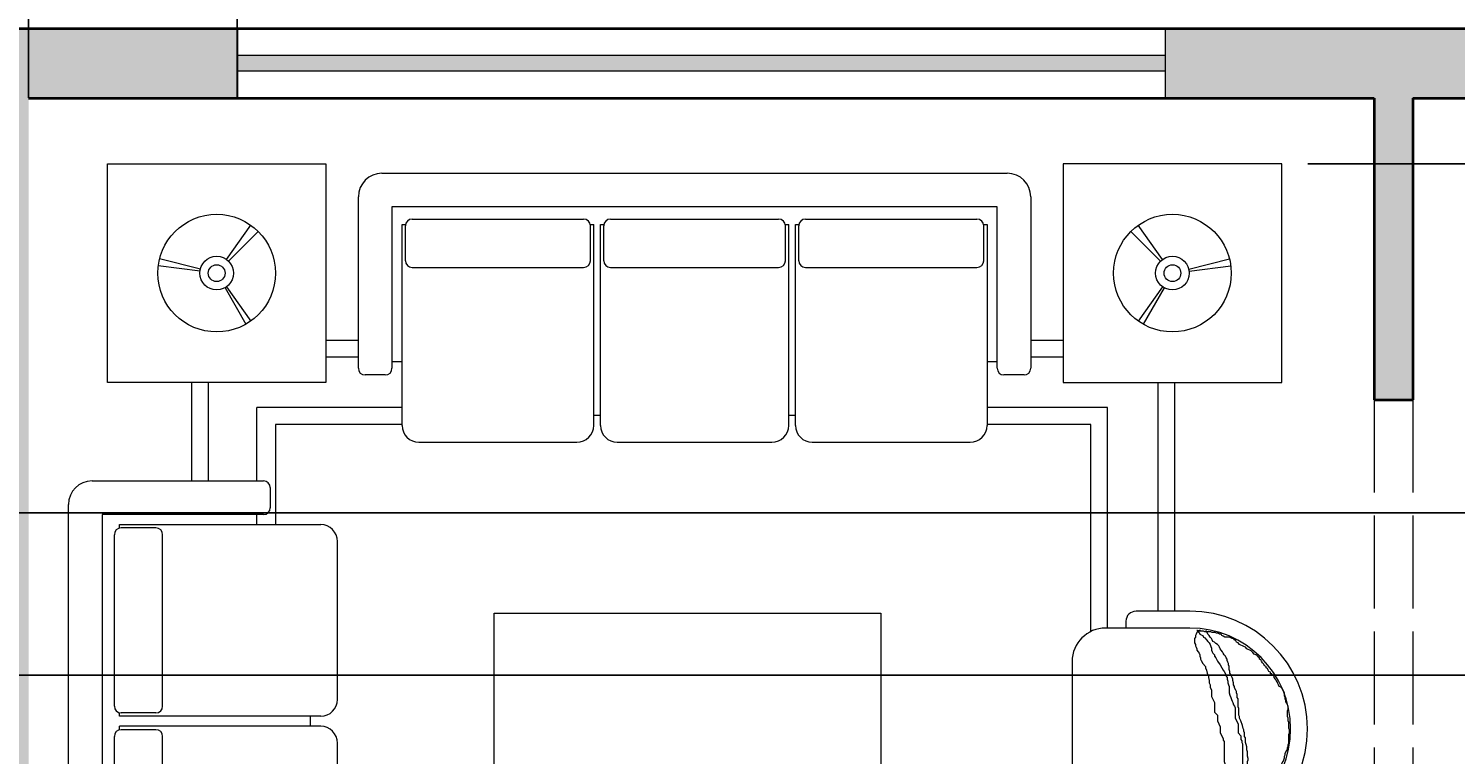
# Model space of a CAD drawing. Units: inches. Extents: x 2330 to 3943, y 1763 to 3461.
# Tile 29 of 40: x 3097 to 3281, y 3069 to 3163. Entities that reach past the tile are written whole.
import ezdxf

# ---------------------------------------------------------------- set-up
doc = ezdxf.new("R2010")
doc.units = ezdxf.units.IN
doc.linetypes.add('ACAD_ISO02W100', pattern=[15, 12, -3])
for name, color, linetype, lineweight in [('A-ANNO-DIMS', 2, 'Continuous', 18), ('A-FURN', 8, 'Continuous', 13), ('A-GLAZ', 4, 'Continuous', 18), ('A-WALL', 7, 'Continuous', 40), ('A-WALL-OVHD', 7, 'ACAD_ISO02W100', 18), ('A-WALL-PATT', 252, 'Continuous', 13)]:
    doc.layers.add(name, color=color, linetype=linetype, lineweight=lineweight)
doc.styles.get("Standard").update_dxf_attribs({"font": 'arial.ttf'})
doc.dimstyles.get("Standard").update_dxf_attribs({"dimtxt": 0.18, "dimasz": 0.18, "dimexe": 0.18, "dimexo": 0.0625, "dimgap": 0.09, "dimtad": 0, "dimtih": 1, "dimtoh": 1, "dimdec": 4, "dimzin": 0, "dimdsep": 46, "dimtxsty": 'Standard', "dimcen": 0.09, "dimadec": 0, "dimazin": 0, "dimtfac": 1, "dimtdec": 4, "dimtofl": 0, "dimtmove": 0, "dimatfit": 3, "dimfxl": 1, "dimtolj": 1, "dimtzin": 0, "dimarcsym": 0})

# ---------------------------------------------------------------- blocks, each defined once
blk = doc.blocks.new('A$C78064EA7')
for p, q in [((932.1, 3320.6), (2792.1, 3320.6)), ((862.1, 2740.6), (862.1, 3250.6)), ((2862.1, 3250.6), (2862.1, 2740.6)), ((962.1, 3220.6), (962.1, 2740.6)), ((2762.1, 3220.6), (962.1, 3220.6)), ((1022.1, 3184.3), (1532.1, 3184.3)), ((1612.1, 3184.3), (2112.1, 3184.3)), ((2192.1, 3184.3), (2702.1, 3184.3)), ((2762.1, 2740.6), (2762.1, 3220.6)), ((469.8, 3064.3), (542.4, 3166)), ((476.1, 3059), (564.4, 3147.3)), ((992.1, 3168.5), (1002.1, 3168.5)), ((992.1, 2570.6), (992.1, 3168.5)), ((1002.1, 3060.6), (1002.1, 3164.3)), ((1551.6, 3168.5), (1562.1, 3168.5)), ((1552.1, 3060.6), (1552.1, 3164.3)), ((1562.1, 2570.6), (1562.1, 3168.5)), ((1582.1, 3168.5), (1592.5, 3168.5)), ((1582.1, 2570.6), (1582.1, 3168.5)), ((1592.1, 3060.6), (1592.1, 3164.3)), ((2131.6, 3168.5), (2142.1, 3168.5)), ((2132.1, 3060.6), (2132.1, 3164.3)), ((2142.1, 2570.6), (2142.1, 3168.5)), ((2162.1, 3168.5), (2172.5, 3168.5)), ((2162.1, 2570.6), (2162.1, 3168.5)), ((2172.1, 3060.6), (2172.1, 3164.3)), ((2721.6, 3168.5), (2732.1, 3168.5)), ((2722.1, 3060.6), (2722.1, 3164.3)), ((2732.1, 3168.5), (2732.1, 2570.6)), ((3248.1, 3059), (3159.7, 3147.3)), ((3254.4, 3064.3), (3181.7, 3166)), ((392.2, 3035.7), (270.9, 3066)), ((3331.9, 3035.7), (3453.2, 3066)), ((391.1, 3029.8), (267.1, 3045.3)), ((1022.1, 3040.6), (1532.1, 3040.6)), ((1612.1, 3040.6), (2112.1, 3040.6)), ((2192.1, 3040.6), (2702.1, 3040.6)), ((3333, 3029.8), (3457.1, 3045.3)), ((465.5, 2980.2), (527.5, 2871.7)), ((469.8, 2982.9), (542.4, 2881.2)), ((3254.4, 2982.9), (3181.7, 2881.2)), ((3258.6, 2980.2), (3196.6, 2871.7)), ((862.1, 2823.6), (765.7, 2823.6)), ((2958.4, 2823.6), (2862.1, 2823.6)), ((862.1, 2773.6), (765.7, 2773.6)), ((962.1, 2760.6), (992.1, 2760.6)), ((2732.1, 2760.6), (2762.1, 2760.6)), ((2958.4, 2773.6), (2862.1, 2773.6)), ((942.1, 2720.6), (882.1, 2720.6)), ((2842.1, 2720.6), (2782.1, 2720.6)), ((365.7, 2698.6), (365.7, 2405.5)), ((415.7, 2698.6), (415.7, 2405.5)), ((3240.7, 2017.9), (3240.7, 2698.6)), ((3290.7, 2017.9), (3290.7, 2698.6)), ((992.1, 2623.6), (560, 2623.6)), ((560, 2405.5), (560, 2623.6)), ((1562.1, 2600.6), (1582.1, 2600.6)), ((2142.1, 2600.6), (2162.1, 2600.6)), ((992.1, 2573.6), (615.7, 2573.6)), ((615.7, 2573.6), (615.7, 2275.5)), ((1042.1, 2520.6), (1512.1, 2520.6)), ((1632.1, 2520.6), (2092.1, 2520.6)), ((2212.1, 2520.6), (2682.1, 2520.6)), ((70, 2405.5), (580, 2405.5)), ((600, 2385.5), (600, 2325.5)), ((0, 1045.5), (0, 2335.5)), ((580, 2305.5), (100, 2305.5)), ((100, 2305.5), (100, 1075.5)), ((560, 2275.5), (560, 2305.5)), ((152.1, 2275.5), (750, 2275.5)), ((152.1, 2265.1), (152.1, 2275.5)), ((260, 2265.5), (156.3, 2265.5)), ((136.3, 1735.5), (136.3, 2245.5)), ((280, 1735.5), (280, 2245.5)), ((800, 1755.5), (800, 2225.5)), ((3335.1, 2017.9), (3175.1, 2017.9)), ((3335.1, 1967.9), (3085.1, 1967.9)), ((3145.1, 1987.9), (3145.1, 1967.9)), ((3358.2, 1958.7), (3353.6, 1950)), ((3358.2, 1961), (3355.9, 1961)), ((3362.5, 1958.7), (3358.2, 1961)), ((3362.5, 1961), (3358.2, 1958.7)), ((3358.2, 1958.7), (3362.5, 1954.4)), ((3366.8, 1961), (3362.5, 1961)), ((3375.5, 1958.7), (3362.5, 1958.7)), ((3362.5, 1954.4), (3364.5, 1950)), ((3380.1, 1956.4), (3375.5, 1958.7)), ((3397.4, 1956.4), (3380.1, 1956.4)), ((3384.4, 1958.7), (3382.1, 1958.7)), ((3386.4, 1954.4), (3384.4, 1958.7)), ((3388.7, 1950), (3386.4, 1954.4)), ((3402, 1954.4), (3397.4, 1956.4)), ((3410.6, 1954.4), (3402, 1954.4)), ((3415, 1952.1), (3410.6, 1954.4)), ((3351.6, 1941.1), (3349.3, 1936.8)), ((3349.3, 1936.8), (3349.3, 1923.5)), ((3349.3, 1923.5), (3351.6, 1919.2)), ((3353.6, 1950), (3351.6, 1945.4)), ((3351.6, 1945.4), (3351.6, 1941.1)), ((3351.6, 1919.2), (3351.6, 1914.9)), ((3351.6, 1914.9), (3353.6, 1910.5)), ((3353.6, 1910.5), (3355.9, 1906.2)), ((3364.5, 1950), (3369.1, 1947.7)), ((3369.1, 1947.7), (3373.5, 1945.4)), ((3373.5, 1945.4), (3375.5, 1941.1)), ((3375.5, 1941.1), (3380.1, 1939.1)), ((3380.1, 1939.1), (3384.4, 1932.4)), ((3384.4, 1932.4), (3388.7, 1928.1)), ((3393.1, 1945.4), (3388.7, 1950)), ((3388.7, 1928.1), (3393.1, 1923.5)), ((3395.4, 1941.1), (3393.1, 1945.4)), ((3393.1, 1923.5), (3395.4, 1919.2)), ((3399.7, 1936.8), (3395.4, 1941.1)), ((3395.4, 1919.2), (3397.4, 1912.5)), ((3397.4, 1912.5), (3399.7, 1908.2)), ((3402, 1932.4), (3399.7, 1936.8)), ((3404, 1928.1), (3402, 1932.4)), ((3408.6, 1925.8), (3404, 1928.1)), ((3412.9, 1921.5), (3408.6, 1925.8)), ((3417.3, 1919.2), (3412.9, 1921.5)), ((3419.6, 1952.1), (3415, 1952.1)), ((3421.6, 1914.9), (3417.3, 1919.2)), ((3423.9, 1950), (3419.6, 1952.1)), ((3423.9, 1910.5), (3421.6, 1914.9)), ((3428.2, 1950), (3423.9, 1950)), ((3425.9, 1906.2), (3423.9, 1910.5)), ((3430.5, 1945.4), (3428.2, 1950)), ((3434.8, 1943.4), (3430.5, 1945.4)), ((3439.2, 1941.1), (3434.8, 1943.4)), ((3452.4, 1941.1), (3439.2, 1941.1)), ((3456.7, 1939.1), (3452.4, 1941.1)), ((3461.1, 1936.8), (3456.7, 1939.1)), ((3465.4, 1936.8), (3461.1, 1936.8)), ((3467.7, 1932.4), (3465.4, 1936.8)), ((3472, 1930.1), (3467.7, 1932.4)), ((3474.3, 1925.8), (3472, 1930.1)), ((3478.7, 1923.5), (3474.3, 1925.8)), ((3483, 1919.2), (3478.7, 1923.5)), ((3487.3, 1917.2), (3483, 1919.2)), ((3491.6, 1914.9), (3487.3, 1917.2)), ((3496.2, 1912.5), (3491.6, 1914.9)), ((3500.6, 1910.5), (3496.2, 1912.5)), ((3504.9, 1906.2), (3500.6, 1910.5)), ((2985.1, 1867.9), (2985.1, 1467.9)), ((3355.9, 1906.2), (3355.9, 1901.6)), ((3355.9, 1901.6), (3360.2, 1897.3)), ((3360.2, 1897.3), (3362.5, 1892.9)), ((3362.5, 1892.9), (3364.5, 1888.6)), ((3364.5, 1888.6), (3364.5, 1884.3)), ((3364.5, 1884.3), (3366.8, 1879.7)), ((3366.8, 1879.7), (3366.8, 1875.3)), ((3366.8, 1875.3), (3369.1, 1871)), ((3369.1, 1871), (3373.5, 1862.3)), ((3399.7, 1908.2), (3399.7, 1901.6)), ((3399.7, 1901.6), (3402, 1897.3)), ((3402, 1897.3), (3404, 1892.9)), ((3404, 1892.9), (3408.6, 1888.6)), ((3408.6, 1888.6), (3408.6, 1884.3)), ((3408.6, 1884.3), (3412.9, 1879.7)), ((3412.9, 1879.7), (3417.3, 1869)), ((3417.3, 1869), (3425.9, 1858)), ((3428.2, 1901.6), (3425.9, 1906.2)), ((3432.5, 1897.3), (3428.2, 1901.6)), ((3434.8, 1892.9), (3432.5, 1897.3)), ((3436.9, 1888.6), (3434.8, 1892.9)), ((3441.5, 1884.3), (3436.9, 1888.6)), ((3443.5, 1879.7), (3441.5, 1884.3)), ((3445.8, 1875.3), (3443.5, 1879.7)), ((3445.8, 1871), (3445.8, 1875.3)), ((3447.8, 1866.7), (3445.8, 1871)), ((3509.2, 1903.9), (3504.9, 1906.2)), ((3513.8, 1901.6), (3509.2, 1903.9)), ((3518.1, 1899.6), (3513.8, 1901.6)), ((3522.5, 1895.2), (3518.1, 1899.6)), ((3526.8, 1890.6), (3522.5, 1895.2)), ((3531.1, 1888.6), (3526.8, 1890.6)), ((3535.7, 1886.3), (3531.1, 1888.6)), ((3537.7, 1882), (3535.7, 1886.3)), ((3542.1, 1879.7), (3537.7, 1882)), ((3542.1, 1875.3), (3542.1, 1879.7)), ((3546.7, 1873.3), (3542.1, 1875.3)), ((3548.7, 1869), (3546.7, 1873.3)), ((3551, 1864.4), (3548.7, 1869)), ((3373.5, 1862.3), (3382.1, 1853.4)), ((3382.1, 1853.4), (3382.1, 1849.1)), ((3382.1, 1849.1), (3384.4, 1842.4)), ((3384.4, 1842.4), (3386.4, 1833.8)), ((3386.4, 1833.8), (3391, 1825.1)), ((3391, 1825.1), (3391, 1820.5)), ((3425.9, 1858), (3430.5, 1849.1)), ((3430.5, 1849.1), (3434.8, 1842.4)), ((3434.8, 1842.4), (3436.9, 1838.1)), ((3436.9, 1838.1), (3441.5, 1831.5)), ((3441.5, 1831.5), (3443.5, 1825.1)), ((3443.5, 1825.1), (3445.8, 1820.5)), ((3450.1, 1862.3), (3447.8, 1866.7)), ((3450.1, 1858), (3450.1, 1862.3)), ((3452.4, 1853.4), (3450.1, 1858)), ((3452.4, 1844.8), (3452.4, 1853.4)), ((3454.4, 1838.1), (3452.4, 1844.8)), ((3454.4, 1833.8), (3454.4, 1838.1)), ((3456.7, 1829.5), (3454.4, 1833.8)), ((3458.8, 1825.1), (3456.7, 1829.5)), ((3461.1, 1820.5), (3458.8, 1825.1)), ((3555.3, 1860), (3551, 1864.4)), ((3557.6, 1855.7), (3555.3, 1860)), ((3561.9, 1853.4), (3557.6, 1855.7)), ((3561.9, 1849.1), (3561.9, 1853.4)), ((3566.3, 1847.1), (3561.9, 1849.1)), ((3568.6, 1842.4), (3566.3, 1847.1)), ((3570.6, 1838.1), (3568.6, 1842.4)), ((3574.9, 1836.1), (3570.6, 1838.1)), ((3574.9, 1831.5), (3574.9, 1836.1)), ((3579.5, 1831.5), (3574.9, 1831.5)), ((3581.5, 1827.2), (3579.5, 1831.5)), ((3585.9, 1825.1), (3581.5, 1827.2)), ((3585.9, 1820.5), (3585.9, 1825.1)), ((3391, 1820.5), (3393.1, 1811.9)), ((3393.1, 1811.9), (3393.1, 1805.2)), ((3393.1, 1805.2), (3395.4, 1798.6)), ((3395.4, 1798.6), (3395.4, 1792.2)), ((3395.4, 1792.2), (3399.7, 1783.3)), ((3399.7, 1783.3), (3399.7, 1763.7)), ((3445.8, 1820.5), (3445.8, 1816.2)), ((3445.8, 1816.2), (3447.8, 1809.6)), ((3447.8, 1809.6), (3447.8, 1805.2)), ((3447.8, 1805.2), (3450.1, 1798.6)), ((3450.1, 1798.6), (3452.4, 1794.3)), ((3452.4, 1794.3), (3452.4, 1774.7)), ((3463.4, 1816.2), (3461.1, 1820.5)), ((3463.4, 1811.9), (3463.4, 1816.2)), ((3465.4, 1805.2), (3463.4, 1811.9)), ((3465.4, 1798.6), (3465.4, 1805.2)), ((3467.7, 1794.3), (3465.4, 1798.6)), ((3467.7, 1789.9), (3467.7, 1794.3)), ((3472, 1783.3), (3467.7, 1789.9)), ((3474.3, 1779), (3472, 1783.3)), ((3590.5, 1816.2), (3585.9, 1820.5)), ((3592.5, 1811.9), (3590.5, 1816.2)), ((3594.8, 1807.5), (3592.5, 1811.9)), ((3596.8, 1803.2), (3594.8, 1807.5)), ((3599.1, 1798.6), (3596.8, 1803.2)), ((3601.4, 1794.3), (3599.1, 1798.6)), ((3605.7, 1792.2), (3601.4, 1794.3)), ((3610.1, 1787.6), (3605.7, 1792.2)), ((3612.4, 1783.3), (3610.1, 1787.6)), ((3614.4, 1779), (3612.4, 1783.3)), ((3399.7, 1763.7), (3408.6, 1746.1)), ((3408.6, 1746.1), (3408.6, 1717.5)), ((3452.4, 1774.7), (3454.4, 1768)), ((3454.4, 1768), (3456.7, 1761.4)), ((3456.7, 1761.4), (3458.8, 1755)), ((3458.8, 1755), (3461.1, 1750.4)), ((3461.1, 1750.4), (3463.4, 1746.1)), ((3463.4, 1746.1), (3465.4, 1739.5)), ((3474.3, 1774.7), (3474.3, 1779)), ((3476.3, 1770.3), (3474.3, 1774.7)), ((3476.3, 1761.4), (3476.3, 1770.3)), ((3478.7, 1757.1), (3476.3, 1761.4)), ((3478.7, 1733.1), (3478.7, 1757.1)), ((3616.7, 1774.7), (3614.4, 1779)), ((3616.7, 1766), (3616.7, 1774.7)), ((3618.7, 1761.4), (3616.7, 1766)), ((3618.7, 1757.1), (3618.7, 1761.4)), ((3621, 1752.7), (3618.7, 1757.1)), ((3621, 1748.4), (3621, 1752.7)), ((3623.3, 1744.1), (3621, 1748.4)), ((3625.3, 1739.5), (3623.3, 1744.1)), ((152.1, 1705.5), (152.1, 1716)), ((750, 1705.5), (152.1, 1705.5)), ((260, 1715.5), (156.3, 1715.5)), ((720, 1685.5), (720, 1705.5)), ((3408.6, 1717.5), (3417.3, 1708.9)), ((3417.3, 1708.9), (3417.3, 1691.3)), ((3465.4, 1739.5), (3467.7, 1735.1)), ((3467.7, 1735.1), (3469.7, 1730.8)), ((3469.7, 1730.8), (3469.7, 1700.2)), ((3469.7, 1700.2), (3478.7, 1682.6)), ((3480.7, 1728.5), (3478.7, 1733.1)), ((3480.7, 1708.9), (3480.7, 1728.5)), ((3483, 1704.6), (3480.7, 1708.9)), ((3483, 1700.2), (3483, 1704.6)), ((3485.3, 1695.6), (3483, 1700.2)), ((3627.6, 1735.1), (3625.3, 1739.5)), ((3625.3, 1722.1), (3627.6, 1726.5)), ((3625.3, 1704.6), (3625.3, 1722.1)), ((3627.6, 1700.2), (3625.3, 1704.6)), ((3627.6, 1726.5), (3627.6, 1735.1)), ((3627.6, 1691.3), (3627.6, 1700.2)), ((750, 1675.5), (152.1, 1675.5)), ((152.1, 1665.1), (152.1, 1675.5)), ((260, 1665.5), (156.3, 1665.5)), ((720, 1675.5), (720, 1695.5)), ((3417.3, 1691.3), (3425.9, 1674)), ((3425.9, 1674), (3425.9, 1656.4)), ((3425.9, 1656.4), (3434.8, 1638.8)), ((3478.7, 1682.6), (3478.7, 1656.4)), ((3478.7, 1656.4), (3487.3, 1647.4)), ((3487.3, 1691.3), (3485.3, 1695.6)), ((3491.6, 1678.3), (3487.3, 1691.3)), ((3493.9, 1669.4), (3491.6, 1678.3)), ((3496.2, 1665), (3493.9, 1669.4)), ((3496.2, 1660.7), (3496.2, 1665)), ((3498.2, 1656.4), (3496.2, 1660.7)), ((3498.2, 1645.4), (3498.2, 1656.4)), ((3629.9, 1687), (3627.6, 1691.3)), ((3629.9, 1669.4), (3629.9, 1687)), ((3632, 1665), (3629.9, 1669.4)), ((3629.9, 1652), (3632, 1656.4)), ((3632, 1656.4), (3632, 1665)), ((136.3, 1135.5), (136.3, 1645.5)), ((280, 1135.5), (280, 1645.5)), ((800, 1155.5), (800, 1625.5)), ((3434.8, 1638.8), (3434.8, 1634.5)), ((3434.8, 1634.5), (3436.9, 1630.1)), ((3436.9, 1630.1), (3436.9, 1571)), ((3487.3, 1647.4), (3487.3, 1636.5)), ((3487.3, 1636.5), (3489.6, 1632.1)), ((3489.6, 1632.1), (3489.6, 1627.8)), ((3489.6, 1627.8), (3491.6, 1623.5)), ((3491.6, 1623.5), (3491.6, 1538.1)), ((3500.6, 1641.1), (3498.2, 1645.4)), ((3500.6, 1627.8), (3500.6, 1641.1)), ((3502.6, 1621.2), (3500.6, 1627.8)), ((3504.9, 1614.5), (3502.6, 1621.2)), ((3504.9, 1605.9), (3504.9, 1614.5)), ((3625.3, 1612.5), (3627.6, 1616.9)), ((3627.6, 1621.2), (3629.9, 1625.5)), ((3627.6, 1616.9), (3627.6, 1621.2)), ((3629.9, 1625.5), (3629.9, 1652)), ((3436.9, 1571), (3439.2, 1564.4)), ((3507.2, 1599.3), (3504.9, 1605.9)), ((3507.2, 1586.3), (3507.2, 1599.3)), ((3509.2, 1579.6), (3507.2, 1586.3)), ((3507.2, 1571), (3509.2, 1575.3)), ((3507.2, 1562), (3507.2, 1571)), ((3509.2, 1575.3), (3509.2, 1579.6)), ((3610.1, 1566.4), (3612.4, 1571)), ((3612.4, 1571), (3614.4, 1575.3)), ((3614.4, 1575.3), (3616.7, 1582)), ((3616.7, 1586.3), (3618.7, 1590.6)), ((3616.7, 1582), (3616.7, 1586.3)), ((3618.7, 1594.9), (3621, 1599.3)), ((3618.7, 1590.6), (3618.7, 1594.9)), ((3621, 1599.3), (3623.3, 1603.9)), ((3623.3, 1603.9), (3625.3, 1608.2)), ((3625.3, 1608.2), (3625.3, 1612.5)), ((3439.2, 1564.4), (3439.2, 1527.1)), ((3491.6, 1538.1), (3489.6, 1529.2)), ((3489.6, 1529.2), (3489.6, 1516.2)), ((3504.9, 1557.7), (3507.2, 1562)), ((3504.9, 1518.2), (3504.9, 1557.7)), ((3590.5, 1527.1), (3594.8, 1529.2)), ((3594.8, 1529.2), (3596.8, 1533.5)), ((3596.8, 1533.5), (3599.1, 1538.1)), ((3599.1, 1538.1), (3601.4, 1542.4)), ((3601.4, 1542.4), (3603.4, 1549.1)), ((3603.4, 1549.1), (3605.7, 1553.4)), ((3605.7, 1553.4), (3607.8, 1557.7)), ((3607.8, 1562), (3610.1, 1566.4)), ((3607.8, 1557.7), (3607.8, 1562)), ((3439.2, 1527.1), (3436.9, 1522.5)), ((3436.9, 1522.5), (3436.9, 1505.2)), ((3436.9, 1505.2), (3439.2, 1500.9)), ((3439.2, 1500.9), (3441.5, 1496.3)), ((3441.5, 1496.3), (3441.5, 1491.9)), ((3441.5, 1491.9), (3443.5, 1487.6)), ((3443.5, 1487.6), (3443.5, 1461.4)), ((3487.3, 1507.2), (3485.3, 1496.3)), ((3485.3, 1496.3), (3485.3, 1479)), ((3489.6, 1516.2), (3487.3, 1511.9)), ((3487.3, 1511.9), (3487.3, 1507.2)), ((3500.6, 1502.9), (3502.6, 1509.5)), ((3500.6, 1476.7), (3500.6, 1502.9)), ((3502.6, 1513.9), (3504.9, 1518.2)), ((3502.6, 1509.5), (3502.6, 1513.9)), ((3548.7, 1485.3), (3551, 1489.9)), ((3551, 1489.9), (3564, 1502.9)), ((3564, 1502.9), (3572.9, 1509.5)), ((3572.9, 1509.5), (3577.2, 1513.9)), ((3577.2, 1513.9), (3581.5, 1516.2)), ((3581.5, 1516.2), (3583.8, 1520.5)), ((3583.8, 1520.5), (3588.2, 1522.5)), ((3588.2, 1522.5), (3590.5, 1527.1)), ((3443.5, 1461.4), (3445.8, 1457)), ((3445.8, 1457), (3445.8, 1448.1)), ((3445.8, 1448.1), (3447.8, 1443.8)), ((3447.8, 1443.8), (3447.8, 1439.4)), ((3483, 1450.4), (3480.7, 1446.1)), ((3480.7, 1446.1), (3480.7, 1437.1)), ((3485.3, 1479), (3483, 1472.3)), ((3483, 1472.3), (3483, 1450.4)), ((3491.6, 1439.4), (3493.9, 1443.8)), ((3493.9, 1450.4), (3496.2, 1454.7)), ((3493.9, 1443.8), (3493.9, 1450.4)), ((3496.2, 1463.4), (3498.2, 1468)), ((3496.2, 1454.7), (3496.2, 1463.4)), ((3498.2, 1472.3), (3500.6, 1476.7)), ((3498.2, 1468), (3498.2, 1472.3)), ((3522.5, 1439.4), (3524.8, 1443.8)), ((3524.8, 1443.8), (3529.1, 1446.1)), ((3529.1, 1446.1), (3531.1, 1450.4)), ((3531.1, 1454.7), (3533.4, 1461.4)), ((3531.1, 1450.4), (3531.1, 1454.7)), ((3533.4, 1461.4), (3535.7, 1465.7)), ((3535.7, 1465.7), (3537.7, 1470)), ((3537.7, 1470), (3540, 1474.3)), ((3540, 1474.3), (3542.1, 1479)), ((3542.1, 1479), (3544.4, 1483.3)), ((3544.4, 1483.3), (3548.7, 1485.3)), ((3447.8, 1439.4), (3450.1, 1435.1)), ((3450.1, 1435.1), (3450.1, 1426.2)), ((3450.1, 1426.2), (3452.4, 1421.8)), ((3452.4, 1421.8), (3456.7, 1417.5)), ((3456.7, 1417.5), (3458.8, 1413.2)), ((3458.8, 1413.2), (3472, 1413.2)), ((3474.3, 1419.8), (3472, 1415.2)), ((3472, 1415.2), (3472, 1413.2)), ((3472, 1413.2), (3476.3, 1410.9)), ((3476.3, 1424.2), (3474.3, 1419.8)), ((3478.7, 1428.5), (3476.3, 1424.2)), ((3476.3, 1410.9), (3480.7, 1413.2)), ((3480.7, 1437.1), (3478.7, 1432.8)), ((3478.7, 1432.8), (3478.7, 1428.5)), ((3480.7, 1413.2), (3485.3, 1415.2)), ((3485.3, 1417.5), (3487.3, 1421.8)), ((3485.3, 1413.2), (3485.3, 1417.5)), ((3485.3, 1415.2), (3489.6, 1417.5)), ((3487.3, 1421.8), (3489.6, 1426.2)), ((3489.6, 1435.1), (3491.6, 1439.4)), ((3489.6, 1426.2), (3489.6, 1435.1)), ((3489.6, 1417.5), (3496.2, 1421.8)), ((3496.2, 1421.8), (3500.6, 1424.2)), ((3500.6, 1424.2), (3504.9, 1426.2)), ((3504.9, 1426.2), (3509.2, 1426.2)), ((3509.2, 1426.2), (3511.5, 1430.5)), ((3511.5, 1430.5), (3515.8, 1430.5)), ((3515.8, 1430.5), (3518.1, 1435.1)), ((3518.1, 1435.1), (3522.5, 1439.4)), ((3335.1, 1367.9), (3085.1, 1367.9)), ((3145.1, 1367.9), (3145.1, 1347.9)), ((3175.1, 1317.9), (3335.1, 1317.9)), ((152.1, 1105.5), (152.1, 1115.5)), ((750, 1105.5), (152.1, 1105.5)), ((260, 1115.5), (156.3, 1115.5)), ((560, 1075.5), (560, 1105.5)), ((100, 1075.5), (580, 1075.5)), ((600, 1055.5), (600, 995.5)), ((580, 975.5), (70, 975.5)), ((2261.5, 700), (1861.5, 700)), ((1761.5, 350), (1761.5, 600)), ((2361.5, 350), (2361.5, 600)), ((1711.5, 510), (1711.5, 350)), ((1761.5, 540), (1741.5, 540)), ((2381.5, 540), (2361.5, 540)), ((2411.5, 350), (2411.5, 510)), ((2227.4, 298.6), (2218.8, 294)), ((2236.1, 300.7), (2227.4, 298.6)), ((2242.7, 303), (2236.1, 300.7)), ((2247, 303), (2242.7, 303)), ((2256, 311.6), (2247, 303)), ((2264.6, 315.9), (2256, 311.6)), ((2269, 318.2), (2264.6, 315.9)), ((2273.3, 318.2), (2269, 318.2)), ((2277.9, 320.5), (2273.3, 318.2)), ((2282.2, 320.5), (2277.9, 320.5)), ((2286.6, 322.6), (2282.2, 320.5)), ((2290.9, 324.9), (2286.6, 322.6)), ((2295.2, 329.2), (2290.9, 324.9)), ((2299.8, 329.2), (2295.2, 329.2)), ((2304.2, 331.5), (2299.8, 329.2)), ((2308.5, 333.5), (2304.2, 331.5)), ((2312.8, 333.5), (2308.5, 333.5)), ((2317.1, 335.8), (2312.8, 333.5)), ((2330.4, 335.8), (2317.1, 335.8)), ((2326.1, 300.7), (2321.8, 296.3)), ((2332.7, 305), (2326.1, 300.7)), ((2334.7, 333.5), (2330.4, 335.8)), ((2334.7, 309.6), (2332.7, 305)), ((2339.1, 333.5), (2334.7, 333.5)), ((2339.1, 311.6), (2334.7, 309.6)), ((2343.7, 331.5), (2339.1, 333.5)), ((2341.4, 315.9), (2339.1, 311.6)), ((2343.7, 320.5), (2341.4, 315.9)), ((2352.3, 326.9), (2343.7, 331.5)), ((2348, 322.6), (2343.7, 320.5)), ((2343.7, 296.3), (2348, 298.6)), ((2352.3, 326.9), (2348, 322.6)), ((2348, 298.6), (2352.3, 300.7)), ((2350, 305), (2352.3, 309.6)), ((2350, 287.7), (2350, 305)), ((2352.3, 322.6), (2354.6, 326.9)), ((2354.6, 322.6), (2352.3, 326.9)), ((2352.3, 309.6), (2352.3, 322.6)), ((2352.3, 300.7), (2352.3, 303)), ((2354.6, 326.9), (2354.6, 329.2)), ((2354.6, 318.2), (2354.6, 322.6)), ((2050, 259.2), (2032.4, 250.2)), ((2067.6, 259.2), (2050, 259.2)), ((2084.9, 267.8), (2067.6, 259.2)), ((2102.5, 267.8), (2084.9, 267.8)), ((2111.2, 276.5), (2102.5, 267.8)), ((2139.7, 276.5), (2111.2, 276.5)), ((2157.3, 285.4), (2139.7, 276.5)), ((2176.9, 285.4), (2157.3, 285.4)), ((2185.9, 289.7), (2176.9, 285.4)), ((2192.2, 289.7), (2185.9, 289.7)), ((2198.9, 292), (2192.2, 289.7)), ((2205.5, 292), (2198.9, 292)), ((2214.2, 294), (2205.5, 292)), ((2218.8, 294), (2214.2, 294)), ((2251.7, 259.2), (2242.7, 254.6)), ((2262.6, 267.8), (2251.7, 259.2)), ((2273.3, 272.1), (2262.6, 267.8)), ((2277.9, 276.5), (2273.3, 272.1)), ((2282.2, 276.5), (2277.9, 276.5)), ((2286.6, 281.1), (2282.2, 276.5)), ((2290.9, 283.1), (2286.6, 281.1)), ((2295.2, 285.4), (2290.9, 283.1)), ((2290.9, 252.5), (2295.2, 256.9)), ((2301.9, 285.4), (2295.2, 285.4)), ((2295.2, 256.9), (2299.8, 259.2)), ((2299.8, 259.2), (2304.2, 261.2)), ((2306.2, 287.7), (2301.9, 285.4)), ((2304.2, 261.2), (2308.5, 263.5)), ((2312.8, 289.7), (2306.2, 287.7)), ((2308.5, 263.5), (2312.8, 267.8)), ((2317.1, 292), (2312.8, 289.7)), ((2312.8, 267.8), (2315.1, 272.1)), ((2315.1, 272.1), (2319.5, 276.5)), ((2321.8, 296.3), (2317.1, 292)), ((2319.5, 276.5), (2321.8, 281.1)), ((2321.8, 281.1), (2326.1, 283.1)), ((2326.1, 283.1), (2330.4, 285.4)), ((2330.4, 285.4), (2334.7, 289.7)), ((2334.7, 289.7), (2339.1, 292)), ((2339.1, 292), (2343.7, 296.3)), ((2339.1, 254.6), (2343.7, 256.9)), ((2343.7, 261.2), (2345.7, 265.5)), ((2343.7, 256.9), (2343.7, 261.2)), ((2345.7, 270.1), (2348, 274.4)), ((2345.7, 265.5), (2345.7, 270.1)), ((2348, 283.1), (2350, 287.7)), ((2348, 274.4), (2348, 283.1)), ((1806.8, 213.1), (1804.5, 208.7)), ((1811.2, 228.3), (1806.8, 226.3)), ((1806.8, 226.3), (1806.8, 213.1)), ((1808.9, 213.1), (1806.8, 213.1)), ((1813.5, 210.7), (1808.9, 213.1)), ((1815.5, 232.7), (1811.2, 228.3)), ((1819.8, 235), (1815.5, 232.7)), ((1828.8, 235), (1819.8, 235)), ((1833.1, 237.3), (1828.8, 235)), ((1837.4, 237.3), (1833.1, 237.3)), ((1841.7, 239.3), (1837.4, 237.3)), ((1850.7, 239.3), (1841.7, 239.3)), ((1855, 241.6), (1850.7, 239.3)), ((1881.3, 241.6), (1855, 241.6)), ((1885.6, 243.6), (1881.3, 241.6)), ((1889.9, 243.6), (1885.6, 243.6)), ((1894.5, 245.9), (1889.9, 243.6)), ((1898.9, 248.2), (1894.5, 245.9)), ((1916.2, 248.2), (1898.9, 248.2)), ((1920.8, 245.9), (1916.2, 248.2)), ((1958, 245.9), (1920.8, 245.9)), ((1964.6, 248.2), (1958, 245.9)), ((2023.8, 248.2), (1964.6, 248.2)), ((2028.1, 250.2), (2023.8, 248.2)), ((2032.4, 250.2), (2028.1, 250.2)), ((2093.9, 215.4), (2076.3, 206.4)), ((2124.4, 215.4), (2093.9, 215.4)), ((2128.8, 217.4), (2124.4, 215.4)), ((2133.1, 219.7), (2128.8, 217.4)), ((2139.7, 221.7), (2133.1, 219.7)), ((2144.1, 224), (2139.7, 221.7)), ((2148.7, 226.3), (2144.1, 224)), ((2155, 228.3), (2148.7, 226.3)), ((2161.7, 230.6), (2155, 228.3)), ((2168.3, 232.7), (2161.7, 230.6)), ((2187.9, 232.7), (2168.3, 232.7)), ((2172.6, 210.7), (2176.9, 213.1)), ((2176.9, 213.1), (2183.6, 217.4)), ((2183.6, 217.4), (2187.9, 217.4)), ((2192.2, 235), (2187.9, 232.7)), ((2187.9, 217.4), (2192.2, 219.7)), ((2198.9, 237.3), (2192.2, 235)), ((2192.2, 219.7), (2198.9, 219.7)), ((2203.2, 237.3), (2198.9, 237.3)), ((2198.9, 219.7), (2205.5, 221.7)), ((2209.8, 239.3), (2203.2, 237.3)), ((2205.5, 221.7), (2209.8, 221.7)), ((2214.2, 239.3), (2209.8, 239.3)), ((2209.8, 221.7), (2214.2, 224)), ((2218.8, 241.6), (2214.2, 239.3)), ((2214.2, 224), (2218.8, 226.3)), ((2225.1, 243.6), (2218.8, 241.6)), ((2218.8, 226.3), (2223.1, 228.3)), ((2223.1, 228.3), (2227.4, 230.6)), ((2231.8, 248.2), (2225.1, 243.6)), ((2227.4, 230.6), (2231.8, 230.6)), ((2236.1, 250.2), (2231.8, 248.2)), ((2231.8, 230.6), (2238.4, 232.7)), ((2242.7, 254.6), (2236.1, 250.2)), ((2238.4, 232.7), (2247, 232.7)), ((2247, 232.7), (2251.7, 235)), ((2251.7, 235), (2256, 235)), ((2256, 235), (2260.3, 237.3)), ((2260.3, 237.3), (2264.6, 239.3)), ((2264.6, 239.3), (2269, 239.3)), ((2269, 239.3), (2273.3, 241.6)), ((2273.3, 241.6), (2277.9, 243.6)), ((2277.9, 243.6), (2282.2, 248.2)), ((2282.2, 248.2), (2286.6, 250.2)), ((2286.6, 250.2), (2290.9, 252.5)), ((2319.5, 210.7), (2323.8, 213.1)), ((2323.8, 213.1), (2326.1, 217.4)), ((2326.1, 217.4), (2330.4, 219.7)), ((2330.4, 224), (2332.7, 228.3)), ((2330.4, 219.7), (2330.4, 224)), ((2332.7, 228.3), (2334.7, 232.7)), ((2334.7, 245.9), (2337.1, 250.2)), ((2334.7, 232.7), (2334.7, 245.9)), ((2337.1, 250.2), (2339.1, 254.6)), ((1804.5, 208.7), (1806.8, 204.4)), ((1806.8, 204.4), (1808.9, 199.8)), ((1806.8, 199.8), (1811.2, 199.8)), ((1808.9, 199.8), (1811.2, 195.5)), ((1811.2, 199.8), (1815.5, 197.8)), ((1811.2, 195.5), (1815.5, 188.8)), ((1817.8, 208.7), (1813.5, 210.7)), ((1815.5, 197.8), (1819.8, 195.5)), ((1815.5, 188.8), (1817.8, 184.5)), ((1822.1, 206.4), (1817.8, 208.7)), ((1817.8, 184.5), (1819.8, 180.2)), ((1819.8, 195.5), (1828.8, 195.5)), ((1819.8, 180.2), (1819.8, 175.9)), ((1819.8, 175.9), (1824.1, 173.6)), ((1826.5, 206.4), (1822.1, 206.4)), ((1824.1, 173.6), (1824.1, 169.2)), ((1830.8, 204.4), (1826.5, 206.4)), ((1828.8, 195.5), (1833.1, 193.5)), ((1839.7, 204.4), (1830.8, 204.4)), ((1833.1, 193.5), (1837.4, 191.2)), ((1837.4, 191.2), (1844, 191.2)), ((1844, 202.1), (1839.7, 204.4)), ((1866, 202.1), (1844, 202.1)), ((1844, 191.2), (1848.4, 188.8)), ((1848.4, 188.8), (1857, 188.8)), ((1857, 188.8), (1861.6, 186.8)), ((1861.6, 186.8), (1866, 186.8)), ((1872.6, 199.8), (1866, 202.1)), ((1866, 186.8), (1870.3, 184.5)), ((1870.3, 184.5), (1896.6, 184.5)), ((1889.9, 199.8), (1872.6, 199.8)), ((1900.9, 197.8), (1889.9, 199.8)), ((1896.6, 184.5), (1903.2, 182.5)), ((1905.5, 197.8), (1900.9, 197.8)), ((1903.2, 182.5), (1907.5, 182.5)), ((1909.8, 195.5), (1905.5, 197.8)), ((1907.5, 182.5), (1911.8, 180.2)), ((1922.8, 195.5), (1909.8, 195.5)), ((1911.8, 180.2), (1951.4, 180.2)), ((1931.7, 193.5), (1922.8, 195.5)), ((2017.1, 193.5), (1931.7, 193.5)), ((1951.4, 180.2), (1955.7, 177.9)), ((1955.7, 177.9), (1964.6, 177.9)), ((1964.6, 177.9), (1969, 175.9)), ((1969, 175.9), (1973.3, 175.9)), ((1973.3, 175.9), (1979.9, 177.9)), ((1979.9, 177.9), (1992.9, 177.9)), ((1992.9, 177.9), (1999.5, 180.2)), ((1999.5, 180.2), (2008.2, 180.2)), ((2008.2, 180.2), (2014.8, 182.5)), ((2014.8, 182.5), (2021.5, 184.5)), ((2021.5, 195.5), (2017.1, 193.5)), ((2025.8, 195.5), (2021.5, 195.5)), ((2021.5, 184.5), (2034.7, 184.5)), ((2030.1, 197.8), (2025.8, 195.5)), ((2041.1, 197.8), (2030.1, 197.8)), ((2034.7, 184.5), (2039.1, 186.8)), ((2039.1, 186.8), (2050, 186.8)), ((2050, 206.4), (2041.1, 197.8)), ((2076.3, 206.4), (2050, 206.4)), ((2050, 186.8), (2054.3, 188.8)), ((2054.3, 188.8), (2058.7, 188.8)), ((2058.7, 188.8), (2063, 191.2)), ((2063, 191.2), (2071.9, 193.5)), ((2071.9, 193.5), (2084.9, 197.8)), ((2084.9, 197.8), (2089.3, 199.8)), ((2089.3, 199.8), (2093.9, 202.1)), ((2093.9, 202.1), (2098.2, 202.1)), ((2098.2, 202.1), (2102.5, 204.4)), ((2102.5, 204.4), (2122.1, 204.4)), ((2122.1, 204.4), (2126.8, 206.4)), ((2126.8, 206.4), (2150.7, 206.4)), ((2150.7, 206.4), (2155, 208.7)), ((2155, 208.7), (2164, 208.7)), ((2164, 208.7), (2168.3, 210.7)), ((2168.3, 210.7), (2172.6, 210.7)), ((2293.2, 166.9), (2295.2, 171.3)), ((2295.2, 171.3), (2297.5, 175.9)), ((2297.5, 175.9), (2299.8, 180.2)), ((2299.8, 180.2), (2304.2, 184.5)), ((2304.2, 184.5), (2306.2, 188.8)), ((2306.2, 188.8), (2308.5, 193.5)), ((2308.5, 193.5), (2310.8, 197.8)), ((2310.8, 197.8), (2312.8, 202.1)), ((2312.8, 202.1), (2317.1, 206.4)), ((2317.1, 206.4), (2319.5, 210.7)), ((1824.1, 169.2), (1828.8, 166.9)), ((1828.8, 166.9), (1833.1, 162.6)), ((1833.1, 162.6), (1837.4, 160.3)), ((1837.4, 160.3), (1839.7, 156)), ((1839.7, 156), (1844, 154)), ((1844, 154), (1848.4, 154)), ((1848.4, 154), (1855, 151.7)), ((1855, 151.7), (1859.3, 149.4)), ((1859.3, 149.4), (1863.7, 147.3)), ((1863.7, 147.3), (1868, 145)), ((1868, 145), (1872.6, 143)), ((1872.6, 143), (1876.9, 140.7)), ((1876.9, 140.7), (1879, 136.4)), ((1879, 136.4), (1883.6, 134.1)), ((1883.6, 134.1), (1896.6, 121.1)), ((2247, 123.1), (2249.4, 127.5)), ((2249.4, 127.5), (2253.7, 129.8)), ((2253.7, 129.8), (2258, 134.1)), ((2258, 134.1), (2262.6, 136.4)), ((2262.6, 136.4), (2267, 138.4)), ((2267, 138.4), (2269, 143)), ((2269, 143), (2273.3, 143)), ((2273.3, 143), (2275.6, 147.3)), ((2275.6, 147.3), (2279.9, 149.4)), ((2279.9, 149.4), (2282.2, 154)), ((2282.2, 154), (2284.3, 158.3)), ((2284.3, 158.3), (2288.9, 162.6)), ((2288.9, 162.6), (2293.2, 166.9)), ((1896.6, 121.1), (1903.2, 112.2)), ((1903.2, 112.2), (1907.5, 107.9)), ((1907.5, 107.9), (1909.8, 103.5)), ((1909.8, 103.5), (1914.1, 101.2)), ((1914.1, 101.2), (1916.2, 96.9)), ((1916.2, 96.9), (1920.8, 94.6)), ((1920.8, 94.6), (1922.8, 90.3)), ((1922.8, 90.3), (1927.1, 88.3)), ((1927.1, 88.3), (1931.7, 86)), ((1931.7, 86), (1936.1, 83.7)), ((2187.9, 83.7), (2192.2, 86)), ((2192.2, 86), (2196.9, 88.3)), ((2196.9, 88.3), (2201.2, 90.3)), ((2201.2, 90.3), (2205.5, 92.6)), ((2205.5, 92.6), (2209.8, 94.6)), ((2209.8, 94.6), (2214.2, 99.2)), ((2214.2, 99.2), (2218.8, 99.2)), ((2218.8, 99.2), (2220.8, 103.5)), ((2220.8, 103.5), (2225.1, 105.6)), ((2225.1, 110.2), (2229.7, 110.2)), ((2225.1, 105.6), (2225.1, 110.2)), ((2229.7, 110.2), (2231.8, 114.5)), ((2231.8, 114.5), (2236.1, 116.5)), ((2236.1, 116.5), (2240.7, 118.8)), ((2240.7, 118.8), (2242.7, 123.1)), ((2242.7, 123.1), (2247, 123.1)), ((1936.1, 83.7), (1942.7, 81.6)), ((1942.7, 81.6), (1947, 79.3)), ((1947, 79.3), (1951.4, 77.3)), ((1951.4, 77.3), (1955.7, 77.3)), ((1955.7, 77.3), (1960, 75)), ((1960, 75), (1964.6, 72.7)), ((1964.6, 72.7), (1969, 70.7)), ((1969, 70.7), (1975.6, 68.4)), ((1975.6, 68.4), (1979.9, 68.4)), ((1979.9, 68.4), (1984.2, 66.4)), ((1984.2, 66.4), (1988.6, 66.4)), ((1988.6, 66.4), (1992.9, 64.1)), ((1992.9, 64.1), (1997.5, 61.8)), ((1997.5, 61.8), (2001.8, 59.7)), ((2001.8, 59.7), (2006.2, 59.7)), ((2006.2, 59.7), (2010.5, 57.4)), ((2010.5, 57.4), (2014.8, 57.4)), ((2014.8, 57.4), (2019.2, 55.1)), ((2019.2, 55.1), (2045.7, 55.1)), ((2045.7, 55.1), (2050, 53.1)), ((2050, 53.1), (2058.7, 53.1)), ((2058.7, 53.1), (2063, 55.1)), ((2063, 55.1), (2080.6, 55.1)), ((2080.6, 55.1), (2084.9, 57.4)), ((2084.9, 57.4), (2093.9, 57.4)), ((2093.9, 57.4), (2098.2, 59.7)), ((2098.2, 59.7), (2115.8, 59.7)), ((2115.8, 59.7), (2120.1, 57.4)), ((2120.1, 57.4), (2128.8, 57.4)), ((2128.8, 57.4), (2133.1, 59.7)), ((2133.1, 59.7), (2137.7, 61.8)), ((2137.7, 61.8), (2142, 64.1)), ((2142, 64.1), (2146.4, 64.1)), ((2146.4, 64.1), (2150.7, 66.4)), ((2150.7, 66.4), (2155, 66.4)), ((2155, 66.4), (2159.6, 68.4)), ((2159.6, 68.4), (2168.3, 68.4)), ((2168.3, 68.4), (2172.6, 70.7)), ((2172.6, 70.7), (2176.9, 72.7)), ((2176.9, 72.7), (2181.3, 75)), ((2181.3, 75), (2185.9, 79.3)), ((2185.9, 79.3), (2187.9, 83.7))]:
    blk.add_line(p, q)
for points in [[(765.7, 2698.6), (115.7, 2698.6), (115.7, 3348.6), (765.7, 3348.6)], [(2958.4, 2698.6), (3608.4, 2698.6), (3608.4, 3348.6), (2958.4, 3348.6)], [(1265.7, 1361.6), (1265.7, 2011.6), (2415.7, 2011.6), (2415.7, 1361.6)]]:
    blk.add_lwpolyline(points, close=True)
for points in [[(3090.7, 1967.9), (3090.7, 2623.6), (2732.1, 2623.6)], [(3040.7, 1957.5), (3040.7, 2573.6), (2732.1, 2573.6)], [(2361.5, 598.6), (3040.7, 598.6), (3040.7, 1378.2)], [(2361.5, 548.6), (3090.7, 548.6), (3090.7, 1367.9)], [(2411.5, 348.6), (3290.7, 348.6), (3290.7, 1317.9)], [(2411.5, 398.6), (3240.7, 398.6), (3240.7, 1317.9)], [(615.7, 1105.5), (615.7, 598.6), (1761.5, 598.6)], [(365.7, 975.5), (365.7, 348.6), (1711.5, 348.6)], [(415.7, 975.5), (415.7, 398.6), (1711.5, 398.6)], [(565.7, 975.5), (565.7, 548.6), (1761.5, 548.6)]]:
    blk.add_lwpolyline(points)
for centre, radius in [((440.7, 3023.6), 175), ((3283.4, 3023.6), 175), ((440.7, 3023.6), 50), ((3283.4, 3023.6), 50), ((440.7, 3023.6), 25), ((3283.4, 3023.6), 25)]:
    blk.add_circle(centre, radius)
for centre, radius, start, end in [((932.1, 3250.6), 70, 90, 180), ((2792.1, 3250.6), 70, 0, 90), ((1022.1, 3164.3), 20, 90, 180), ((1532.1, 3164.3), 20, 0, 90), ((1612.1, 3164.3), 20, 90, 180), ((2112.1, 3164.3), 20, 0, 90), ((2192.1, 3164.3), 20, 90, 180), ((2702.1, 3164.3), 20, 0, 90), ((1022.1, 3060.6), 20, 180, 270), ((1532.1, 3060.6), 20, 270, 0), ((1612.1, 3060.6), 20, 180, 270), ((2112.1, 3060.6), 20, 270, 0), ((2192.1, 3060.6), 20, 180, 270), ((2702.1, 3060.6), 20, 270, 0), ((882.1, 2740.6), 20, 180, 270), ((942.1, 2740.6), 20, 270, 0), ((2782.1, 2740.6), 20, 180, 270), ((2842.1, 2740.6), 20, 270, 0), ((1042.1, 2570.6), 50, 180, 270), ((1512.1, 2570.6), 50, 270, 0), ((1632.1, 2570.6), 50, 180, 270), ((2092.1, 2570.6), 50, 270, 0), ((2212.1, 2570.6), 50, 180, 270), ((2682.1, 2570.6), 50, 270, 0), ((70, 2335.5), 70, 90, 180), ((580, 2385.5), 20, 0, 90), ((580, 2325.5), 20, 270, 0), ((156.3, 2245.5), 20, 90, 180), ((260, 2245.5), 20, 0, 90), ((750, 2225.5), 50, 0, 90), ((3175.1, 1987.9), 30, 90, 180), ((3335.1, 1667.9), 350, 270, 90), ((3085.1, 1867.9), 100, 90, 180), ((3335.1, 1667.9), 300, 270, 90), ((750, 1755.5), 50, 270, 0), ((156.3, 1735.5), 20, 180, 270), ((260, 1735.5), 20, 270, 0), ((156.3, 1645.5), 20, 90, 180), ((260, 1645.5), 20, 0, 90), ((750, 1625.5), 50, 0, 90), ((3085.1, 1467.9), 100, 180, 270), ((3175.1, 1347.9), 30, 180, 270), ((750, 1155.5), 50, 270, 0), ((156.3, 1135.5), 20, 180, 270), ((260, 1135.5), 20, 270, 0), ((580, 1055.5), 20, 0, 90), ((70, 1045.5), 70, 180, 270), ((580, 995.5), 20, 270, 0), ((1861.5, 600), 100, 90, 180), ((2261.5, 600), 100, 0, 90), ((1741.5, 510), 30, 90, 180), ((2381.5, 510), 30, 0, 90), ((2061.5, 350), 350, 180, 0), ((2061.5, 350), 300, 180, 360)]:
    blk.add_arc(centre, radius, start, end)
blk = doc.blocks.new('WINDOW-120IN')
h = blk.add_hatch(color=256)
h.dxf.hatch_style = 1
h.paths.add_polyline_path([(120, 5.5), (0, 5.5), (0, 3.5), (120, 3.5)])
for p, q in [((0, 9), (0, 0)), ((120, 9), (120, 0)), ((120, 5.5), (0, 5.5)), ((120, 3.5), (0, 3.5))]:
    blk.add_line(p, q)
blk = doc.blocks.new('*D48')
at = {"layer": 'A-ANNO-DIMS', "color": 0, "lineweight": -2, "transparency": 16777216}
for p, q in [((3262.1, 3145.15), (3286.25, 3145.15)), ((3286.07, 3144.97), (3286.07, 3072.54)), ((3286.07, 2999.75), (3286.07, 3072.18)), ((3262.1, 2999.57), (3286.25, 2999.57))]:
    blk.add_line(p, q, dxfattribs=at)
at = {"layer": 'A-ANNO-DIMS', "color": 0, "transparency": 16777216}
for points in [[(3286.04, 3144.97), (3286.1, 3144.97), (3286.07, 3145.15)], [(3286.04, 2999.75), (3286.1, 2999.75), (3286.07, 2999.57)]]:
    blk.add_solid(points, dxfattribs=at)
at = {"layer": 'Defpoints', "color": 0, "transparency": 16777216}
for p in [(3262.04, 3145.15), (3286.07, 3145.15), (3262.04, 2999.57)]:
    blk.add_point(p, dxfattribs=at)
at = {"layer": 'A-ANNO-DIMS', "color": 0, "transparency": 16777216, "insert": (3286.07, 3072.36), "char_height": 0.18, "attachment_point": 5}
blk.add_mtext('\\A1;146', dxfattribs=at)
blk = doc.blocks.new('*D86')
at = {"layer": 'A-ANNO-DIMS', "color": 0, "lineweight": -2, "transparency": 16777216}
for p, q in [((2979.18, 3100.04), (3942.54, 3100.04)), ((3942.36, 3099.86), (3942.36, 3089.72)), ((3942.36, 3079.22), (3942.36, 3089.36)), ((2979.18, 3079.04), (3942.54, 3079.04))]:
    blk.add_line(p, q, dxfattribs=at)
at = {"layer": 'A-ANNO-DIMS', "color": 0, "transparency": 16777216}
for points in [[(3942.33, 3099.86), (3942.39, 3099.86), (3942.36, 3100.04)], [(3942.33, 3079.22), (3942.39, 3079.22), (3942.36, 3079.04)]]:
    blk.add_solid(points, dxfattribs=at)
at = {"layer": 'Defpoints', "color": 0, "transparency": 16777216}
for p in [(2979.12, 3100.04), (2979.12, 3079.04), (3942.36, 3079.04)]:
    blk.add_point(p, dxfattribs=at)
at = {"layer": 'A-ANNO-DIMS', "color": 0, "transparency": 16777216, "insert": (3942.36, 3089.54), "char_height": 0.18, "attachment_point": 5}
blk.add_mtext('\\A1;21', dxfattribs=at)
blk = doc.blocks.new('*D94')
at = {"layer": 'A-ANNO-DIMS', "color": 0, "lineweight": -2, "transparency": 16777216}
for p, q in [((3096.66, 3153.71), (3096.66, 3461.3)), ((3096.84, 3461.12), (3109.94, 3461.12)), ((3123.48, 3461.12), (3110.38, 3461.12)), ((3123.66, 3153.71), (3123.66, 3461.3))]:
    blk.add_line(p, q, dxfattribs=at)
at = {"layer": 'A-ANNO-DIMS', "color": 0, "transparency": 16777216}
for points in [[(3096.84, 3461.15), (3096.84, 3461.09), (3096.66, 3461.12)], [(3123.48, 3461.15), (3123.48, 3461.09), (3123.66, 3461.12)]]:
    blk.add_solid(points, dxfattribs=at)
at = {"layer": 'Defpoints', "color": 0, "transparency": 16777216}
for p in [(3123.66, 3461.12), (3096.66, 3153.65), (3123.66, 3153.65)]:
    blk.add_point(p, dxfattribs=at)
at = {"layer": 'A-ANNO-DIMS', "color": 0, "transparency": 16777216, "insert": (3110.16, 3461.12), "char_height": 0.18, "attachment_point": 5}
blk.add_mtext('\\A1;27', dxfattribs=at)

msp = doc.modelspace()

# ---------------------------------------------------------------- hatches: boundary and pattern name
at = {"layer": 'A-WALL-PATT'}
h = msp.add_hatch(color=256, dxfattribs=at)
h.dxf.hatch_style = 1
h.paths.add_polyline_path([(3123.6605, 3162.6524), (3046.6605, 3162.6524), (3046.6605, 3153.6524), (3091.6605, 3153.6524), (3091.6605, 3003.6524), (3087.6605, 3003.6524), (3087.6605, 2998.6524), (3091.6605, 2998.6524), (3091.6605, 2994.6524), (3096.6605, 2994.6524), (3096.6605, 3153.6524), (3123.6605, 3153.6524)])
h = msp.add_hatch(color=256, dxfattribs=at)
h.dxf.hatch_style = 1
h.paths.add_polyline_path([(3455.6605, 3162.6524), (3243.6605, 3162.6524), (3243.6605, 3153.6524), (3270.6605, 3153.6524), (3270.6605, 3114.6524), (3275.6605, 3114.6524), (3275.6605, 3153.6524), (3446.6605, 3153.6524), (3446.6605, 3114.6524), (3455.6605, 3114.6524)])

# ---------------------------------------------------------------- linework, layer by layer
at = {"layer": 'A-WALL'}
for p, q in [((2968.6605, 3162.6524), (3455.6605, 3162.6524)), ((3096.6605, 3153.6524), (3270.6605, 3153.6524)), ((3270.6605, 3153.6524), (3270.6605, 3114.6524)), ((3275.6605, 3153.6524), (3275.6605, 3114.6524)), ((3275.6605, 3153.6524), (3446.6605, 3153.6524)), ((3270.6605, 3114.6524), (3275.6605, 3114.6524))]:
    msp.add_line(p, q, dxfattribs=at)
at = {"layer": 'A-WALL-OVHD'}
for p, q in [((3270.6605, 3114.6524), (3270.6605, 3018.6524)), ((3275.6605, 3114.6524), (3275.6605, 3018.6524))]:
    msp.add_line(p, q, dxfattribs=at)

# ---------------------------------------------------------------- block references
at = {"layer": 'A-FURN', "xscale": 0.0434754410177484, "yscale": 0.0434754410177484, "zscale": 0.0434754410177484}
msp.add_blockref('A$C78064EA7', (3101.8308, 2999.5664), dxfattribs=at)
at = {"layer": 'A-GLAZ'}
msp.add_blockref('WINDOW-120IN', (3123.6605, 3153.6524), dxfattribs=at)

# ---------------------------------------------------------------- dimensions: what is measured, and where the dimension line sits
at = {"layer": 'A-ANNO-DIMS'}
dim = msp.add_linear_dim(base=(3123.6605, 3461.1231), p1=(3096.6605, 3153.6524), p2=(3123.6605, 3153.6524), dimstyle='Standard', override={"dimdec": 0, "dimlfac": 1, "dimrnd": 0, "dimzin": 0, "dimdsep": 46, "dimlunit": 2}, dxfattribs=at)
dim.commit()
dim.dimension.update_dxf_attribs({"geometry": '*D94', "text_midpoint": (3110.1605, 3461.1231)})
for base, p1, p2, picture, middle in [((3286.0727, 3145.1485), (3262.0412, 2999.5664), (3262.0412, 3145.1485), '*D48', (3286.0727, 3072.3575)), ((3942.361, 3079.0386), (2979.1218, 3100.0386), (2979.1218, 3079.0386), '*D86', (3942.361, 3089.5386))]:
    dim = msp.add_linear_dim(base=base, p1=p1, p2=p2, angle=90, dimstyle='Standard', override={"dimdec": 0, "dimlfac": 1, "dimrnd": 0, "dimzin": 0, "dimdsep": 46, "dimlunit": 2}, dxfattribs=at)
    dim.commit()
    dim.dimension.update_dxf_attribs({"geometry": picture, "text_midpoint": middle})

doc.saveas('drawing.dxf')
